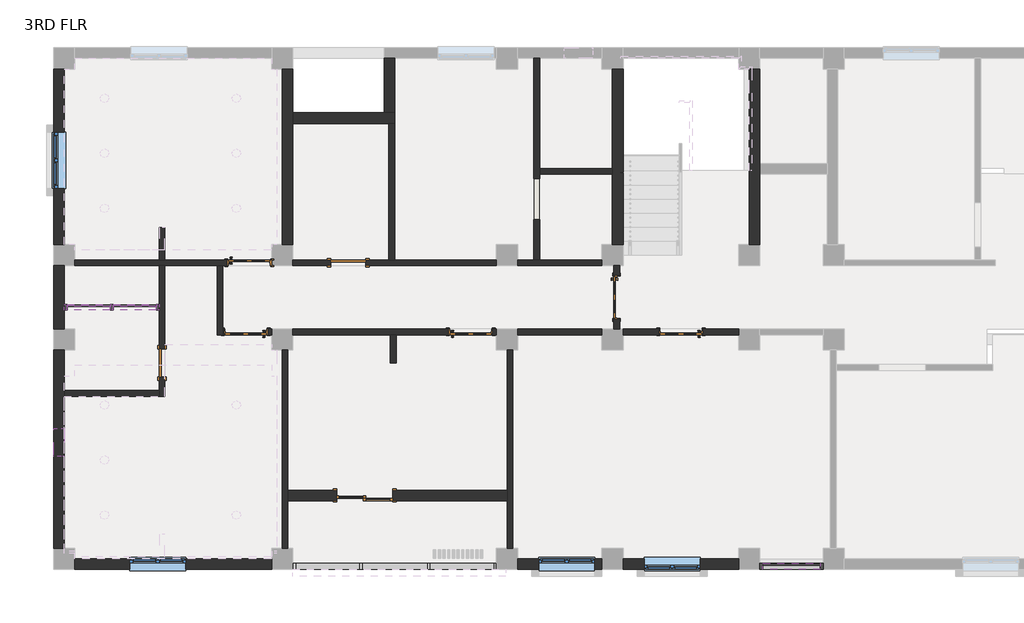
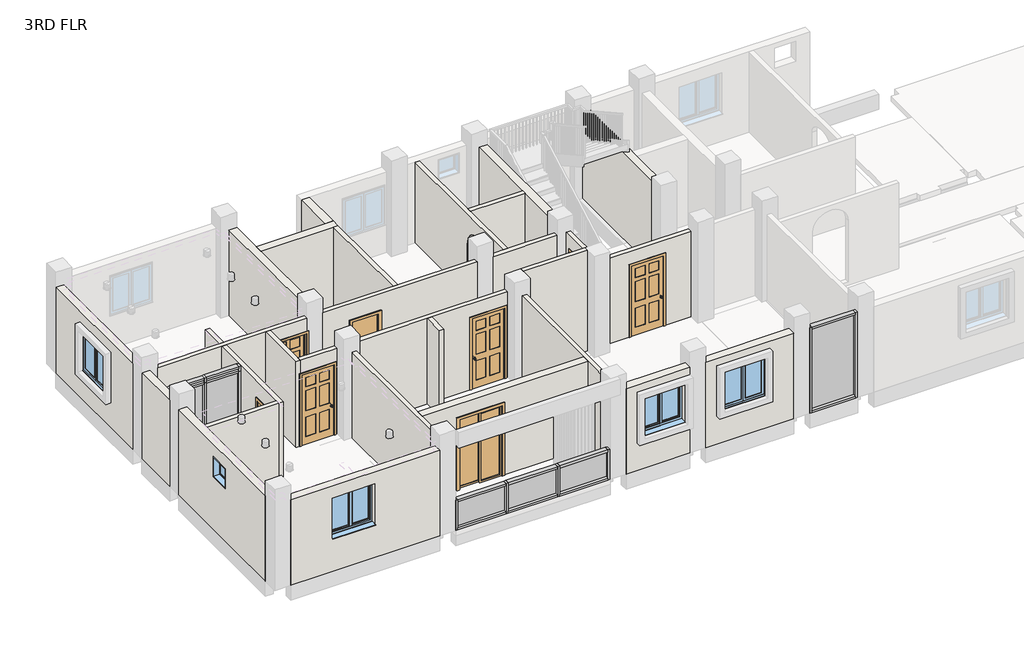
# One storey, part 1 of 5: 29 walls, 26 members, 8 doors, 8 plates, 5 windows.
"""IFC4 building model written with IfcOpenShell, lengths in millimetres."""

from ifc_helpers import new_model, si_unit, point, frame, origin, place, context, project, spatial, polyline, ellipse_curve, trimmed, outline, extrude, faceted_brep, transform, mapped, element, save
from ifc_brep_helpers import plane_surface, extruded_surface, advanced_brep
from components import door_double_sliding_4436dcad, door_c610b25b, door_03e3dfb5, single_flush_2_x_7_bath_room_door_025d1c86, door_e00f436c, member_f0fea5a5, member_f6f0dfdd, member_ee409385, member_876f8f00, member_2b4cd6f1, member_0dc43c0c, member_51239652, member_c58de4df, member_410c6227, member_73c23c35, member_71eb4692, member_9f3fc137, system_panel_glazed_e8343dfa, system_panel_glazed_58efc156, system_panel_glazed_69a0d9e9, system_panel_glazed_27716cba, system_panel_glazed_7ffa2d15, window_80340324, w2_0001_4_x_4_window_9dec5fc7

model = new_model("IFC4")

# Units and contexts
model_context = context("Model", 3, world=origin())
ifc_project = project(units=[si_unit("LENGTHUNIT", "METRE", prefix="MILLI")], contexts=[model_context])

# Site, building, storey
site = spatial("IfcSite", under=ifc_project)
building = spatial("IfcBuilding", under=site)
storey = spatial("IfcBuildingStorey", under=building, Name="3RD FLR", Elevation=9448.8)

# Doors
placement = place(None, origin())
door_double_sliding_shape = door_double_sliding_4436dcad(model_context)
element("IfcDoor", 1, ObjectType="Door-Double-Sliding", at=placement, inside=storey, context=model_context, shape_type="MappedRepresentation", body=[
    mapped(door_double_sliding_shape, transform((-8630.2456086, -9389.2679047, 9448.8), x_axis=(-1.0, 0.0, 0.0), y_axis=(0.0, -1.0, 0.0), z_axis=(0.0, 0.0, 1.0))),
])
door_shape = door_c610b25b(model_context)
element("IfcDoor", 2, ObjectType="Door-Interior-Single-6_Panel-Wood : 36\" x 84\"", at=placement, inside=storey, context=model_context, shape_type="MappedRepresentation", body=[
    mapped(door_shape, transform((-6331.5456086, -5967.8544704, 9448.8), x_axis=(1.0, 0.0, 0.0), y_axis=(0.0, 1.0, 0.0), z_axis=(0.0, 0.0, 1.0))),
])
element("IfcDoor", 3, ObjectType="Door-Interior-Single-6_Panel-Wood : 36\" x 84\"", at=placement, inside=storey, context=model_context, shape_type="MappedRepresentation", body=[
    mapped(door_shape, transform((-3172.4206086, -5215.3794704, 9448.8), x_axis=(0.0, -1.0, 0.0), y_axis=(1.0, 0.0, 0.0), z_axis=(0.0, 0.0, 1.0))),
])
door_2_shape = door_03e3dfb5(model_context)
element("IfcDoor", 4, ObjectType="Door-Interior-Single-6_Panel-Wood : 36\" x 84\"", at=placement, inside=storey, context=model_context, shape_type="MappedRepresentation", body=[
    mapped(door_2_shape, transform((-11207.742897, -5967.8544704, 9448.8), x_axis=(-1.0, 0.0, 0.0), y_axis=(0.0, -1.0, 0.0), z_axis=(0.0, 0.0, 1.0))),
])
element("IfcDoor", 5, ObjectType="Door-Interior-Single-6_Panel-Wood : 36\" x 84\"", at=placement, inside=storey, context=model_context, shape_type="MappedRepresentation", body=[
    mapped(door_2_shape, transform((-11132.1456086, -4462.9044704, 9448.8), x_axis=(1.0, 0.0, 0.0), y_axis=(0.0, 1.0, 0.0), z_axis=(0.0, 0.0, 1.0))),
])
element("IfcDoor", 6, ObjectType="Door-Interior-Single-6_Panel-Wood : 36\" x 84\"", at=placement, inside=storey, context=model_context, shape_type="MappedRepresentation", body=[
    mapped(door_2_shape, transform((-1773.9769742, -5967.8544704, 9448.8), x_axis=(-1.0, 0.0, 0.0), y_axis=(0.0, -1.0, 0.0), z_axis=(0.0, 0.0, 1.0))),
])
single_flush_2_x_7_bath_room_door_shape = single_flush_2_x_7_bath_room_door_025d1c86(model_context)
element("IfcDoor", 7, ObjectType="Single-Flush : 2' X 7' BATH ROOM DOOR", at=placement, inside=storey, context=model_context, shape_type="MappedRepresentation", body=[
    mapped(single_flush_2_x_7_bath_room_door_shape, transform((-13023.2401855, -6639.2659448, 9448.8), x_axis=(0.0, 1.0, 0.0), y_axis=(-1.0, 0.0, 0.0), z_axis=(0.0, 0.0, 1.0))),
])
door_3_shape = door_e00f436c(model_context)
element("IfcDoor", 8, ObjectType="Single-Flush : bathroom 2'6\" door", at=placement, inside=storey, context=model_context, shape_type="MappedRepresentation", body=[
    mapped(door_3_shape, transform((-8985.8456086, -4466.0794704, 9448.8), x_axis=(-1.0, 0.0, 0.0), y_axis=(0.0, -1.0, 0.0), z_axis=(0.0, 0.0, 1.0))),
])

# Members
member_shape = member_f0fea5a5(model_context)
element("IfcMember", 9, ObjectType="Rectangular Mullion : 2.5\" x 5\" rectangular", at=placement, inside=storey, context=model_context, shape_type="MappedRepresentation", body=[
    mapped(member_shape, transform((-14116.042897, -5431.2794704, 9448.8), x_axis=(1.0, 0.0, 0.0), y_axis=(0.0, -1.0, 0.0), z_axis=(0.0, 0.0, -1.0))),
])
member_2_shape = member_f6f0dfdd(model_context)
element("IfcMember", 10, ObjectType="Rectangular Mullion : 2.5\" x 5\" rectangular", at=placement, inside=storey, context=model_context, shape_type="MappedRepresentation", body=[
    mapped(member_2_shape, transform((-14116.042897, -5431.2794704, 11887.2), x_axis=(1.0, 0.0, 0.0), y_axis=(0.0, -1.0, 0.0), z_axis=(0.0, 0.0, -1.0))),
])
member_3_shape = member_ee409385(model_context)
element("IfcMember", 11, ObjectType="Rectangular Mullion : 2.5\" x 5\" rectangular", at=placement, inside=storey, context=model_context, shape_type="MappedRepresentation", body=[
    mapped(member_3_shape, transform((-13086.7401855, -5431.2794704, 9448.8), x_axis=(1.0, 0.0, 0.0), y_axis=(0.0, -1.0, 0.0), z_axis=(0.0, 0.0, -1.0))),
])
member_4_shape = member_876f8f00(model_context)
element("IfcMember", 12, ObjectType="Rectangular Mullion : 2.5\" x 5\" rectangular", at=placement, inside=storey, context=model_context, shape_type="MappedRepresentation", body=[
    mapped(member_4_shape, transform((-15145.3456086, -5431.2794704, 12039.6), x_axis=(-1.0, 0.0, 0.0), y_axis=(0.0, -1.0, 0.0), z_axis=(0.0, 0.0, 1.0))),
])
element("IfcMember", 13, ObjectType="Rectangular Mullion : 2.5\" x 5\" rectangular", at=placement, inside=storey, context=model_context, shape_type="MappedRepresentation", body=[
    mapped(member_4_shape, transform((-13086.7401855, -5431.2794704, 11887.2), x_axis=(1.0, 0.0, 0.0), y_axis=(0.0, -1.0, 0.0), z_axis=(0.0, 0.0, -1.0))),
])
element("IfcMember", 14, ObjectType="Rectangular Mullion : 2.5\" x 5\" rectangular", at=placement, inside=storey, context=model_context, shape_type="MappedRepresentation", body=[
    mapped(member_3_shape, transform((-15145.3456086, -5431.2794704, 11887.2), x_axis=(-1.0, 0.0, 0.0), y_axis=(0.0, -1.0, 0.0), z_axis=(0.0, 0.0, 1.0))),
])
member_5_shape = member_2b4cd6f1(model_context)
element("IfcMember", 15, ObjectType="Rectangular Mullion : 2.5\" x 5\" rectangular", at=placement, inside=storey, context=model_context, shape_type="MappedRepresentation", body=[
    mapped(member_5_shape, transform((-5836.2456086, -11052.9679047, 10363.2), x_axis=(0.0, 0.0, 1.0), y_axis=(0.0, -1.0, 0.0), z_axis=(1.0, 0.0, 0.0))),
])
element("IfcMember", 16, ObjectType="Rectangular Mullion : 2.5\" x 5\" rectangular", at=placement, inside=storey, context=model_context, shape_type="MappedRepresentation", body=[
    mapped(member_5_shape, transform((-8750.8956085, -11052.9679047, 10363.2), x_axis=(0.0, 0.0, 1.0), y_axis=(0.0, -1.0, 0.0), z_axis=(1.0, 0.0, 0.0))),
])
element("IfcMember", 17, ObjectType="Rectangular Mullion : 2.5\" x 5\" rectangular", at=placement, inside=storey, context=model_context, shape_type="MappedRepresentation", body=[
    mapped(member_5_shape, transform((-10128.8456086, -11052.9679047, 9448.8), x_axis=(0.0, 0.0, -1.0), y_axis=(0.0, -1.0, 0.0), z_axis=(-1.0, 0.0, 0.0))),
])
element("IfcMember", 18, ObjectType="Rectangular Mullion : 2.5\" x 5\" rectangular", at=placement, inside=storey, context=model_context, shape_type="MappedRepresentation", body=[
    mapped(member_5_shape, transform((-7214.1956087, -11052.9679047, 9448.8), x_axis=(0.0, 0.0, -1.0), y_axis=(0.0, -1.0, 0.0), z_axis=(-1.0, 0.0, 0.0))),
])
member_6_shape = member_0dc43c0c(model_context)
element("IfcMember", 19, ObjectType="Rectangular Mullion : 2.5\" x 5\" rectangular", at=placement, inside=storey, context=model_context, shape_type="MappedRepresentation", body=[
    mapped(member_6_shape, transform((-7277.6956087, -11052.9679047, 10363.2), x_axis=(0.0, 0.0, 1.0), y_axis=(0.0, -1.0, 0.0), z_axis=(1.0, 0.0, 0.0))),
])
element("IfcMember", 20, ObjectType="Rectangular Mullion : 2.5\" x 5\" rectangular", at=placement, inside=storey, context=model_context, shape_type="MappedRepresentation", body=[
    mapped(member_6_shape, transform((-8687.3956085, -11052.9679047, 9448.8), x_axis=(0.0, 0.0, -1.0), y_axis=(0.0, -1.0, 0.0), z_axis=(-1.0, 0.0, 0.0))),
])
member_7_shape = member_51239652(model_context)
element("IfcMember", 21, ObjectType="Rectangular Mullion : 2.5\" x 5\" rectangular", at=placement, inside=storey, context=model_context, shape_type="MappedRepresentation", body=[
    mapped(member_7_shape, transform((-13150.2401855, -5431.2794704, 12039.6), x_axis=(0.0, 0.0, 1.0), y_axis=(0.0, -1.0, 0.0), z_axis=(1.0, 0.0, 0.0))),
])
element("IfcMember", 22, ObjectType="Rectangular Mullion : 2.5\" x 5\" rectangular", at=placement, inside=storey, context=model_context, shape_type="MappedRepresentation", body=[
    mapped(member_7_shape, transform((-14147.792897, -5431.2794704, 12039.6), x_axis=(0.0, 0.0, 1.0), y_axis=(0.0, -1.0, 0.0), z_axis=(1.0, 0.0, 0.0))),
])
element("IfcMember", 23, ObjectType="Rectangular Mullion : 2.5\" x 5\" rectangular", at=placement, inside=storey, context=model_context, shape_type="MappedRepresentation", body=[
    mapped(member_7_shape, transform((-15081.8456086, -5431.2794704, 9448.8), x_axis=(0.0, 0.0, -1.0), y_axis=(0.0, -1.0, 0.0), z_axis=(-1.0, 0.0, 0.0))),
])
element("IfcMember", 24, ObjectType="Rectangular Mullion : 2.5\" x 5\" rectangular", at=placement, inside=storey, context=model_context, shape_type="MappedRepresentation", body=[
    mapped(member_7_shape, transform((-14084.292897, -5431.2794704, 9448.8), x_axis=(0.0, 0.0, -1.0), y_axis=(0.0, -1.0, 0.0), z_axis=(-1.0, 0.0, 0.0))),
])
member_8_shape = member_c58de4df(model_context)
element("IfcMember", 25, ObjectType="Rectangular Mullion : 2.5\" x 5\" rectangular", at=placement, inside=storey, context=model_context, shape_type="MappedRepresentation", body=[
    mapped(member_8_shape, transform((-14147.792897, -5431.2794704, 11887.2), x_axis=(0.0, 0.0, 1.0), y_axis=(0.0, -1.0, 0.0), z_axis=(1.0, 0.0, 0.0))),
])
element("IfcMember", 26, ObjectType="Rectangular Mullion : 2.5\" x 5\" rectangular", at=placement, inside=storey, context=model_context, shape_type="MappedRepresentation", body=[
    mapped(member_8_shape, transform((-13150.2401855, -5431.2794704, 11887.2), x_axis=(0.0, 0.0, 1.0), y_axis=(0.0, -1.0, 0.0), z_axis=(1.0, 0.0, 0.0))),
])
member_9_shape = member_410c6227(model_context)
element("IfcMember", 27, ObjectType="Rectangular Mullion : 2.5\" x 5\" rectangular", at=placement, inside=storey, context=model_context, shape_type="MappedRepresentation", body=[
    mapped(member_9_shape, transform((-8719.1456085, -11052.9679047, 9448.8), x_axis=(1.0, 0.0, 0.0), y_axis=(0.0, -1.0, 0.0), z_axis=(0.0, 0.0, -1.0))),
])
element("IfcMember", 28, ObjectType="Rectangular Mullion : 2.5\" x 5\" rectangular", at=placement, inside=storey, context=model_context, shape_type="MappedRepresentation", body=[
    mapped(member_9_shape, transform((-7245.9456087, -11052.9679047, 9448.8), x_axis=(1.0, 0.0, 0.0), y_axis=(0.0, -1.0, 0.0), z_axis=(0.0, 0.0, -1.0))),
])
member_10_shape = member_73c23c35(model_context)
element("IfcMember", 29, ObjectType="Rectangular Mullion : 2.5\" x 5\" rectangular", at=placement, inside=storey, context=model_context, shape_type="MappedRepresentation", body=[
    mapped(member_10_shape, transform((-5772.7456086, -11052.9679047, 9448.8), x_axis=(1.0, 0.0, 0.0), y_axis=(0.0, -1.0, 0.0), z_axis=(0.0, 0.0, -1.0))),
])
element("IfcMember", 30, ObjectType="Rectangular Mullion : 2.5\" x 5\" rectangular", at=placement, inside=storey, context=model_context, shape_type="MappedRepresentation", body=[
    mapped(member_10_shape, transform((-10192.3456086, -11052.9679047, 10363.2), x_axis=(-1.0, 0.0, 0.0), y_axis=(0.0, -1.0, 0.0), z_axis=(0.0, 0.0, 1.0))),
])
member_11_shape = member_71eb4692(model_context)
element("IfcMember", 31, ObjectType="Rectangular Mullion : 2.5\" x 5\" rectangular", at=placement, inside=storey, context=model_context, shape_type="MappedRepresentation", body=[
    mapped(member_11_shape, transform((1246.8916602, -11052.9679047, 12039.6), x_axis=(0.0, 0.0, 1.0), y_axis=(0.0, -1.0, 0.0), z_axis=(1.0, 0.0, 0.0))),
])
element("IfcMember", 32, ObjectType="Rectangular Mullion : 2.5\" x 5\" rectangular", at=placement, inside=storey, context=model_context, shape_type="MappedRepresentation", body=[
    mapped(member_11_shape, transform((2.2916602, -11052.9679047, 9448.8), x_axis=(0.0, 0.0, -1.0), y_axis=(0.0, -1.0, 0.0), z_axis=(-1.0, 0.0, 0.0))),
])
member_12_shape = member_9f3fc137(model_context)
element("IfcMember", 33, ObjectType="Rectangular Mullion : 2.5\" x 5\" rectangular", at=placement, inside=storey, context=model_context, shape_type="MappedRepresentation", body=[
    mapped(member_12_shape, transform((1310.3916602, -11052.9679047, 9448.8), x_axis=(1.0, 0.0, 0.0), y_axis=(0.0, -1.0, 0.0), z_axis=(0.0, 0.0, -1.0))),
])
element("IfcMember", 34, ObjectType="Rectangular Mullion : 2.5\" x 5\" rectangular", at=placement, inside=storey, context=model_context, shape_type="MappedRepresentation", body=[
    mapped(member_12_shape, transform((-61.2083398, -11052.9679047, 12039.6), x_axis=(-1.0, 0.0, 0.0), y_axis=(0.0, -1.0, 0.0), z_axis=(0.0, 0.0, 1.0))),
])

# Plates
system_panel_glazed_shape = system_panel_glazed_e8343dfa(model_context)
element("IfcPlate", 35, ObjectType="System Panel : Glazed", at=placement, inside=storey, context=model_context, shape_type="MappedRepresentation", body=[
    mapped(system_panel_glazed_shape, transform((-14614.8192528, -5431.2794704, 9512.3), x_axis=(1.0, 0.0, 0.0), y_axis=(0.0, 1.0, 0.0), z_axis=(0.0, 0.0, 1.0))),
])
element("IfcPlate", 36, ObjectType="System Panel : Glazed", at=placement, inside=storey, context=model_context, shape_type="MappedRepresentation", body=[
    mapped(system_panel_glazed_shape, transform((-13617.2665413, -5431.2794704, 9512.3), x_axis=(1.0, 0.0, 0.0), y_axis=(0.0, 1.0, 0.0), z_axis=(0.0, 0.0, 1.0))),
])
system_panel_glazed_2_shape = system_panel_glazed_58efc156(model_context)
element("IfcPlate", 37, ObjectType="System Panel : Glazed", at=placement, inside=storey, context=model_context, shape_type="MappedRepresentation", body=[
    mapped(system_panel_glazed_2_shape, transform((-14614.8192528, -5431.2794704, 11918.95), x_axis=(1.0, 0.0, 0.0), y_axis=(0.0, 1.0, 0.0), z_axis=(0.0, 0.0, 1.0))),
])
element("IfcPlate", 38, ObjectType="System Panel : Glazed", at=placement, inside=storey, context=model_context, shape_type="MappedRepresentation", body=[
    mapped(system_panel_glazed_2_shape, transform((-13617.2665413, -5431.2794704, 11918.95), x_axis=(1.0, 0.0, 0.0), y_axis=(0.0, 1.0, 0.0), z_axis=(0.0, 0.0, 1.0))),
])
system_panel_glazed_3_shape = system_panel_glazed_69a0d9e9(model_context)
element("IfcPlate", 39, ObjectType="System Panel : Glazed", at=placement, inside=storey, context=model_context, shape_type="MappedRepresentation", body=[
    mapped(system_panel_glazed_3_shape, transform((-9439.8706086, -11052.9679047, 9512.3), x_axis=(1.0, 0.0, 0.0), y_axis=(0.0, 1.0, 0.0), z_axis=(0.0, 0.0, 1.0))),
])
element("IfcPlate", 40, ObjectType="System Panel : Glazed", at=placement, inside=storey, context=model_context, shape_type="MappedRepresentation", body=[
    mapped(system_panel_glazed_3_shape, transform((-6525.2206087, -11052.9679047, 9512.3), x_axis=(1.0, 0.0, 0.0), y_axis=(0.0, 1.0, 0.0), z_axis=(0.0, 0.0, 1.0))),
])
system_panel_glazed_4_shape = system_panel_glazed_27716cba(model_context)
element("IfcPlate", 41, ObjectType="System Panel : Glazed", at=placement, inside=storey, context=model_context, shape_type="MappedRepresentation", body=[
    mapped(system_panel_glazed_4_shape, transform((-7982.5456086, -11052.9679047, 9512.3), x_axis=(1.0, 0.0, 0.0), y_axis=(0.0, 1.0, 0.0), z_axis=(0.0, 0.0, 1.0))),
])
system_panel_glazed_5_shape = system_panel_glazed_7ffa2d15(model_context)
element("IfcPlate", 42, ObjectType="System Panel : Glazed", at=placement, inside=storey, context=model_context, shape_type="MappedRepresentation", body=[
    mapped(system_panel_glazed_5_shape, transform((624.5916602, -11052.9679047, 9512.3), x_axis=(1.0, 0.0, 0.0), y_axis=(0.0, 1.0, 0.0), z_axis=(0.0, 0.0, 1.0))),
])

# Walls
element("IfcWall", 43, ObjectType="EXTERIOR WALL 9\"", at=placement, inside=storey, context=model_context, shape_type="SweptSolid", body=[
    extrude(outline(polyline([(9448.8, -14916.7456086), (9448.8, -10649.5456086), (12039.6, -10649.5456086), (12039.6, -14916.7456086), (9448.8, -14916.7456086)]), holes=[polyline([(10448.8, -12503.7456086), (10448.8, -13722.9456086), (11668.0, -13722.9456086), (11668.0, -12503.7456086), (10448.8, -12503.7456086)])]), frame((0.0, -11116.4679047, 0.0), z_axis=(0.0, 1.0, 0.0), x_axis=(0.0, 0.0, 1.0)), (0.0, 0.0, 1.0), 228.6),
])
element("IfcWall", 44, ObjectType="EXTERIOR WALL 9\"", at=placement, inside=storey, context=model_context, shape_type="SweptSolid", body=[
    extrude(outline(polyline([(9448.8, -5315.5456086), (9448.8, -3486.7456086), (12039.6, -3486.7456086), (12039.6, -5315.5456086), (9448.8, -5315.5456086)]), holes=[polyline([(10448.8, -3639.1456086), (10448.8, -4858.3456086), (11668.0, -4858.3456086), (11668.0, -3639.1456086), (10448.8, -3639.1456086)])]), frame((0.0, -11116.4679047, 0.0), z_axis=(0.0, 1.0, 0.0), x_axis=(0.0, 0.0, 1.0)), (0.0, 0.0, 1.0), 228.6),
])
element("IfcWall", 45, ObjectType="EXTERIOR WALL 9\"", at=placement, inside=storey, context=model_context, shape_type="SweptSolid", body=[
    extrude(outline(polyline([(9448.8, -3029.5456086), (9448.8, -518.4083398), (12039.6, -518.4083398), (12039.6, -3029.5456086), (9448.8, -3029.5456086)]), holes=[polyline([(10448.8, -2572.3456086), (11668.0, -2572.3456086), (11668.0, -1353.1456086), (10448.8, -1353.1456086), (10448.8, -2572.3456086)])]), frame((0.0, -11116.4679047, 0.0), z_axis=(0.0, 1.0, 0.0), x_axis=(0.0, 0.0, 1.0)), (0.0, 0.0, 1.0), 228.6),
])
element("IfcWall", 46, ObjectType="EXTERIOR WALL 9\"", at=placement, inside=storey, context=model_context, shape_type="Brep", body=[
    faceted_brep([(-15145.3456086, -10659.2679047, 9448.8), (-15145.3456086, -7363.1659448, 9448.8), (-15145.3456086, -7236.1659448, 9448.8), (-15145.3456086, -6358.3794704, 9448.8), (-15145.3456086, -6358.3794704, 12039.6), (-15145.3456086, -7236.1659448, 12039.6), (-15145.3456086, -7363.1659448, 12039.6), (-15145.3456086, -10659.2679047, 12039.6), (-15145.3456086, -8671.2659448, 11655.8263913), (-15145.3456086, -8061.6659448, 11655.8263913), (-15145.3456086, -8061.6659448, 11046.2263913), (-15145.3456086, -8671.2659448, 11046.2263913), (-15373.9456086, -10659.2679047, 9448.8), (-15373.9456086, -10659.2679047, 12039.6), (-15373.9456086, -6358.3794704, 12039.6), (-15373.9456086, -6358.3794704, 9448.8), (-15373.9456086, -8671.2659448, 11655.8263913), (-15373.9456086, -8671.2659448, 11046.2263913), (-15373.9456086, -8061.6659448, 11046.2263913), (-15373.9456086, -8061.6659448, 11655.8263913)], [[[0, 1, 2, 3, 4, 5, 6, 7], [8, 9, 10, 11]], [[12, 13, 14, 15], [16, 17, 18, 19]], [[3, 2, 1, 0, 12, 15]], [[4, 3, 15, 14]], [[7, 6, 5, 4, 14, 13]], [[0, 7, 13, 12]], [[17, 16, 8, 11]], [[18, 17, 11, 10]], [[19, 18, 10, 9]], [[16, 19, 9, 8]]]),
])
element("IfcWall", 47, ObjectType="EXTERIOR WALL 9\"", at=placement, inside=storey, context=model_context, shape_type="SweptSolid", body=[
    extrude(outline(polyline([(-15145.3456086, -4529.5794704), (-15145.3456086, -5901.1794704), (-15373.9456086, -5901.1794704), (-15373.9456086, -4529.5794704), (-15145.3456086, -4529.5794704)])), frame((0.0, 0.0, 9448.8), z_axis=(0.0, 0.0, 1.0), x_axis=(1.0, 0.0, 0.0)), (0.0, 0.0, 1.0), 2590.8),
])
element("IfcWall", 48, ObjectType="EXTERIOR WALL 9\"", at=placement, inside=storey, context=model_context, shape_type="SweptSolid", body=[
    extrude(outline(polyline([(-262.3794704, 9448.8), (-4072.3794704, 9448.8), (-4072.3794704, 12039.6), (-262.3794704, 12039.6), (-262.3794704, 9448.8)]), holes=[polyline([(-1633.9794704, 10363.2), (-1633.9794704, 11582.4), (-2853.1794704, 11582.4), (-2853.1794704, 10363.2), (-1633.9794704, 10363.2)])]), frame((-15373.9456086, 0.0, 0.0), z_axis=(1.0, 0.0, 0.0), x_axis=(0.0, 1.0, 0.0)), (0.0, 0.0, 1.0), 228.6),
])
element("IfcWall", 49, ObjectType="EXTERIOR WALL 9\"", at=placement, inside=storey, context=model_context, shape_type="Brep", body=[
    faceted_brep([(-10420.9456086, -262.3794704, 9448.8), (-10420.9456086, -4072.3794704, 9448.8), (-10420.9456086, -4072.3794704, 12039.6), (-10420.9456086, -262.3794704, 12039.6), (-10192.3456086, -262.3794704, 9448.8), (-10192.3456086, -262.3794704, 12039.6), (-10192.3456086, -1214.8794704, 12039.6), (-10192.3456086, -1443.4794704, 12039.6), (-10192.3456086, -4072.3794704, 12039.6), (-10192.3456086, -4072.3794704, 9448.8), (-10192.3456086, -1443.4794704, 9448.8), (-10192.3456086, -1214.8794704, 9448.8)], [[[0, 1, 2, 3]], [[4, 5, 6, 7, 8, 9, 10, 11]], [[1, 0, 4, 11, 10, 9]], [[2, 1, 9, 8]], [[3, 2, 8, 7, 6, 5]], [[0, 3, 5, 4]]]),
])
element("IfcWall", 50, ObjectType="EXTERIOR WALL 9\"", at=placement, inside=storey, context=model_context, shape_type="SweptSolid", body=[
    extrude(outline(polyline([(9448.8, -10293.9456086), (9448.8, -9239.8456086), (11582.4, -9239.8456086), (11582.4, -8020.6456086), (9448.8, -8020.6456086), (9448.8, -5544.1456086), (12039.6, -5544.1456086), (12039.6, -10293.9456086), (9448.8, -10293.9456086)])), frame((0.0, -9630.5679047, 0.0), z_axis=(0.0, 1.0, 0.0), x_axis=(0.0, 0.0, 1.0)), (0.0, 0.0, 1.0), 228.6),
])
element("IfcWall", 51, ObjectType="EXTERIOR WALL 9\"", at=placement, inside=storey, context=model_context, shape_type="Brep", body=[
    faceted_brep([(-10192.3456086, -1443.4794704, 9448.8), (-8109.5456086, -1443.4794704, 9448.8), (-7982.5456086, -1443.4794704, 9448.8), (-7982.5456086, -1443.4794704, 12039.6), (-8109.5456086, -1443.4794704, 12039.6), (-10192.3456086, -1443.4794704, 12039.6), (-10192.3456086, -1214.8794704, 9448.8), (-10192.3456086, -1214.8794704, 12039.6), (-8211.1456086, -1214.8794704, 12039.6), (-7982.5456086, -1214.8794704, 12039.6), (-7982.5456086, -1214.8794704, 9448.8), (-8211.1456086, -1214.8794704, 9448.8)], [[[0, 1, 2, 3, 4, 5]], [[6, 7, 8, 9, 10, 11]], [[2, 1, 0, 6, 11, 10]], [[5, 4, 3, 9, 8, 7]], [[0, 5, 7, 6]], [[3, 2, 10, 9]]]),
])
element("IfcWall", 52, ObjectType="EXTERIOR WALL 9\"", at=placement, inside=storey, context=model_context, shape_type="SweptSolid", body=[
    extrude(outline(polyline([(-7982.5456086, -33.7794704), (-7982.5456086, -1214.8794704), (-8211.1456086, -1214.8794704), (-8211.1456086, -33.7794704), (-7982.5456086, -33.7794704)])), frame((0.0, 0.0, 9448.8), z_axis=(0.0, 0.0, 1.0), x_axis=(1.0, 0.0, 0.0)), (0.0, 0.0, 1.0), 2590.8),
])
element("IfcWall", 53, ObjectType="EXTERIOR WALL 9\"", at=placement, inside=storey, context=model_context, shape_type="Brep", body=[
    faceted_brep([(-3258.1456086, -262.3794704, 9448.8), (-3258.1456086, -2421.3794704, 9448.8), (-3258.1456086, -2548.3794704, 9448.8), (-3258.1456086, -4072.3794704, 9448.8), (-3258.1456086, -4072.3794704, 12039.6), (-3258.1456086, -2548.3794704, 12039.6), (-3258.1456086, -2421.3794704, 12039.6), (-3258.1456086, -262.3794704, 12039.6), (-3029.5456086, -262.3794704, 9448.8), (-3029.5456086, -262.3794704, 12039.6), (-3029.5456086, -4072.3794704, 12039.6), (-3029.5456086, -4072.3794704, 9448.8)], [[[0, 1, 2, 3, 4, 5, 6, 7]], [[8, 9, 10, 11]], [[3, 2, 1, 0, 8, 11]], [[4, 3, 11, 10]], [[7, 6, 5, 4, 10, 9]], [[0, 7, 9, 8]]]),
])
element("IfcWall", 54, ObjectType="EXTERIOR WALL 9\"", at=placement, inside=storey, context=model_context, shape_type="Brep", body=[
    faceted_brep([(-289.8083398, -262.3794704, 9448.8), (-289.8083398, -4072.3794704, 9448.8), (-289.8083398, -4072.3794704, 12039.6), (-289.8083398, -262.3794704, 12039.6), (-61.2083398, -262.3794704, 9448.8), (-61.2083398, -262.3794704, 12039.6), (-61.2083398, -2319.7794704, 12039.6), (-61.2083398, -2548.3794704, 12039.6), (-61.2083398, -4072.3794704, 12039.6), (-61.2083398, -4072.3794704, 9448.8), (-61.2083398, -2548.3794704, 9448.8), (-61.2083398, -2319.7794704, 9448.8)], [[[0, 1, 2, 3]], [[4, 5, 6, 7, 8, 9, 10, 11]], [[1, 0, 4, 11, 10, 9]], [[2, 1, 9, 8]], [[3, 2, 8, 7, 6, 5]], [[0, 3, 5, 4]]]),
])
element("IfcWall", 55, ObjectType="INTERIOR WALL 5\"", at=placement, inside=storey, context=model_context, shape_type="Brep", body=[
    faceted_brep([(-10649.5456086, -4529.5794704, 12039.6), (-11702.4401855, -4529.5794704, 12039.6), (-11829.4401855, -4529.5794704, 12039.6), (-12959.7401855, -4529.5794704, 12039.6), (-13086.7401855, -4529.5794704, 12039.6), (-14916.7456086, -4529.5794704, 12039.6), (-14916.7456086, -4529.5794704, 9448.8), (-13086.7401855, -4529.5794704, 9448.8), (-12959.7401855, -4529.5794704, 9448.8), (-11829.4401855, -4529.5794704, 9448.8), (-11702.4401855, -4529.5794704, 9448.8), (-11614.7456086, -4529.5794704, 9448.8), (-11614.7456086, -4529.5794704, 11607.8), (-10649.5456086, -4529.5794704, 11607.8), (-14916.7456086, -4402.5794704, 12039.6), (-13086.7401855, -4402.5794704, 12039.6), (-12959.7401855, -4402.5794704, 12039.6), (-10649.5456086, -4402.5794704, 12039.6), (-10649.5456086, -4402.5794704, 11607.8), (-11614.7456086, -4402.5794704, 11607.8), (-11614.7456086, -4402.5794704, 9448.8), (-12959.7401855, -4402.5794704, 9448.8), (-13086.7401855, -4402.5794704, 9448.8), (-14916.7456086, -4402.5794704, 9448.8)], [[[0, 1, 2, 3, 4, 5, 6, 7, 8, 9, 10, 11, 12, 13]], [[14, 15, 16, 17, 18, 19, 20, 21, 22, 23]], [[6, 23, 22, 21, 20, 11, 10, 9, 8, 7]], [[17, 0, 13, 18]], [[5, 4, 3, 2, 1, 0, 17, 16, 15, 14]], [[6, 5, 14, 23]], [[12, 19, 18, 13]], [[19, 12, 11, 20]]]),
])
element("IfcWall", 56, ObjectType="INTERIOR WALL 5\"", at=placement, inside=storey, context=model_context, shape_type="Brep", body=[
    faceted_brep([(-13086.7401855, -3705.5659448, 12039.6), (-13086.7401855, -3705.5659448, 9448.8), (-13086.7401855, -4402.5794704, 9448.8), (-13086.7401855, -4402.5794704, 12039.6), (-12959.7401855, -3705.5659448, 9448.8), (-12959.7401855, -3705.5659448, 12039.6), (-12959.7401855, -4402.5794704, 12039.6), (-12959.7401855, -4402.5794704, 9448.8)], [[[0, 1, 2, 3]], [[4, 5, 6, 7]], [[1, 4, 7, 2]], [[5, 0, 3, 6]], [[1, 0, 5, 4]], [[3, 2, 7, 6]]]),
    faceted_brep([(-13086.7401855, -7363.1659448, 9448.8), (-13086.7401855, -7363.1659448, 12039.6), (-13086.7401855, -7236.1659448, 12039.6), (-13086.7401855, -4529.5794704, 12039.6), (-13086.7401855, -4529.5794704, 9448.8), (-13086.7401855, -6334.4659448, 9448.8), (-13086.7401855, -6334.4659448, 11480.8), (-13086.7401855, -6944.0659448, 11480.8), (-13086.7401855, -6944.0659448, 9448.8), (-13086.7401855, -7236.1659448, 9448.8), (-12959.7401855, -7363.1659448, 12039.6), (-12959.7401855, -7363.1659448, 9448.8), (-12959.7401855, -6944.0659448, 9448.8), (-12959.7401855, -6944.0659448, 11480.8), (-12959.7401855, -6334.4659448, 11480.8), (-12959.7401855, -6334.4659448, 9448.8), (-12959.7401855, -4529.5794704, 9448.8), (-12959.7401855, -4529.5794704, 12039.6)], [[[0, 1, 2, 3, 4, 5, 6, 7, 8, 9]], [[10, 11, 12, 13, 14, 15, 16, 17]], [[11, 0, 9, 8, 12]], [[15, 5, 4, 16]], [[1, 10, 17, 3, 2]], [[4, 3, 17, 16]], [[1, 0, 11, 10]], [[6, 5, 15, 14]], [[7, 6, 14, 13]], [[8, 7, 13, 12]]]),
])
element("IfcWall", 57, ObjectType="INTERIOR WALL 5\"", at=placement, inside=storey, context=model_context, shape_type="SweptSolid", body=[
    extrude(outline(polyline([(-15145.3456086, -7236.1659448), (-13086.7401855, -7236.1659448), (-13086.7401855, -7363.1659448), (-15145.3456086, -7363.1659448), (-15145.3456086, -7236.1659448)])), frame((0.0, 0.0, 9448.8), z_axis=(0.0, 0.0, 1.0), x_axis=(1.0, 0.0, 0.0)), (0.0, 0.0, 1.0), 2590.8),
])
element("IfcWall", 58, ObjectType="INTERIOR WALL 5\"", at=placement, inside=storey, context=model_context, shape_type="Brep", body=[
    faceted_brep([(-10293.9456086, -10659.2679047, 9448.8), (-10293.9456086, -9630.5679047, 9448.8), (-10293.9456086, -9401.9679047, 9448.8), (-10293.9456086, -6358.3794704, 9448.8), (-10293.9456086, -6358.3794704, 12039.6), (-10293.9456086, -9401.9679047, 12039.6), (-10293.9456086, -9630.5679047, 12039.6), (-10293.9456086, -10659.2679047, 12039.6), (-10420.9456086, -10659.2679047, 9448.8), (-10420.9456086, -10659.2679047, 12039.6), (-10420.9456086, -6358.3794704, 12039.6), (-10420.9456086, -6358.3794704, 9448.8)], [[[0, 1, 2, 3, 4, 5, 6, 7]], [[8, 9, 10, 11]], [[3, 2, 1, 0, 8, 11]], [[4, 3, 11, 10]], [[7, 6, 5, 4, 10, 9]], [[0, 7, 9, 8]]]),
])
element("IfcWall", 59, ObjectType="INTERIOR WALL 5\"", at=placement, inside=storey, context=model_context, shape_type="Brep", body=[
    faceted_brep([(-10192.3456086, -5901.1794704, 9448.8), (-10192.3456086, -5901.1794704, 12039.6), (-5772.7456086, -5901.1794704, 12039.6), (-5772.7456086, -5901.1794704, 9448.8), (-5848.9456086, -5901.1794704, 9448.8), (-5848.9456086, -5901.1794704, 11607.8), (-6814.1456086, -5901.1794704, 11607.8), (-6814.1456086, -5901.1794704, 9448.8), (-10192.3456086, -6028.1794704, 12039.6), (-10192.3456086, -6028.1794704, 9448.8), (-8071.4456086, -6028.1794704, 9448.8), (-7944.4456086, -6028.1794704, 9448.8), (-6814.1456086, -6028.1794704, 9448.8), (-6814.1456086, -6028.1794704, 11607.8), (-5848.9456086, -6028.1794704, 11607.8), (-5848.9456086, -6028.1794704, 9448.8), (-5772.7456086, -6028.1794704, 9448.8), (-5772.7456086, -6028.1794704, 12039.6), (-7944.4456086, -6028.1794704, 12039.6), (-8071.4456086, -6028.1794704, 12039.6)], [[[0, 1, 2, 3, 4, 5, 6, 7]], [[8, 9, 10, 11, 12, 13, 14, 15, 16, 17, 18, 19]], [[9, 0, 7, 12, 11, 10]], [[3, 16, 15, 4]], [[1, 0, 9, 8]], [[2, 1, 8, 19, 18, 17]], [[3, 2, 17, 16]], [[14, 5, 4, 15]], [[5, 14, 13, 6]], [[6, 13, 12, 7]]]),
])
element("IfcWall", 60, ObjectType="INTERIOR WALL 5\"", at=placement, inside=storey, context=model_context, shape_type="SweptSolid", body=[
    extrude(outline(polyline([(-8071.4456086, -6637.7794704), (-8071.4456086, -6028.1794704), (-7944.4456086, -6028.1794704), (-7944.4456086, -6637.7794704), (-8071.4456086, -6637.7794704)])), frame((0.0, 0.0, 9448.8), z_axis=(0.0, 0.0, 1.0), x_axis=(1.0, 0.0, 0.0)), (0.0, 0.0, 1.0), 2590.8),
])
element("IfcWall", 61, ObjectType="INTERIOR WALL 5\"", at=placement, inside=storey, context=model_context, shape_type="Brep", body=[
    faceted_brep([(-5417.1456086, -10659.2679047, 9448.8), (-5417.1456086, -6358.3794704, 9448.8), (-5417.1456086, -6358.3794704, 12039.6), (-5417.1456086, -10659.2679047, 12039.6), (-5544.1456086, -10659.2679047, 9448.8), (-5544.1456086, -10659.2679047, 12039.6), (-5544.1456086, -9630.5679047, 12039.6), (-5544.1456086, -9401.9679047, 12039.6), (-5544.1456086, -6358.3794704, 12039.6), (-5544.1456086, -6358.3794704, 9448.8), (-5544.1456086, -9401.9679047, 9448.8), (-5544.1456086, -9630.5679047, 9448.8)], [[[0, 1, 2, 3]], [[4, 5, 6, 7, 8, 9, 10, 11]], [[1, 0, 4, 11, 10, 9]], [[2, 1, 9, 8]], [[3, 2, 8, 7, 6, 5]], [[0, 3, 5, 4]]]),
])
element("IfcWall", 62, ObjectType="INTERIOR WALL 5\"", at=placement, inside=storey, context=model_context, shape_type="Brep", body=[
    faceted_brep([(-10192.3456086, -4529.5794704, 9448.8), (-9366.8456086, -4529.5794704, 9448.8), (-9366.8456086, -4529.5794704, 11480.8), (-8604.8456086, -4529.5794704, 11480.8), (-8604.8456086, -4529.5794704, 9448.8), (-5772.7456086, -4529.5794704, 9448.8), (-5772.7456086, -4529.5794704, 12039.6), (-10192.3456086, -4529.5794704, 12039.6), (-9366.8456086, -4402.5794704, 11480.8), (-9366.8456086, -4402.5794704, 9448.8), (-10192.3456086, -4402.5794704, 9448.8), (-10192.3456086, -4402.5794704, 12039.6), (-8109.5456086, -4402.5794704, 12039.6), (-7982.5456086, -4402.5794704, 12039.6), (-5772.7456086, -4402.5794704, 12039.6), (-5772.7456086, -4402.5794704, 9448.8), (-7982.5456086, -4402.5794704, 9448.8), (-8109.5456086, -4402.5794704, 9448.8), (-8604.8456086, -4402.5794704, 9448.8), (-8604.8456086, -4402.5794704, 11480.8)], [[[0, 1, 2, 3, 4, 5, 6, 7]], [[8, 9, 10, 11, 12, 13, 14, 15, 16, 17, 18, 19]], [[10, 9, 1, 0]], [[18, 17, 16, 15, 5, 4]], [[6, 5, 15, 14]], [[7, 6, 14, 13, 12, 11]], [[0, 7, 11, 10]], [[2, 1, 9, 8]], [[3, 2, 8, 19]], [[4, 3, 19, 18]]]),
])
element("IfcWall", 63, ObjectType="INTERIOR WALL 5\"", at=placement, inside=storey, context=model_context, shape_type="Brep", body=[
    faceted_brep([(-5315.5456086, -4529.5794704, 9448.8), (-3486.7456086, -4529.5794704, 9448.8), (-3486.7456086, -4529.5794704, 12039.6), (-5315.5456086, -4529.5794704, 12039.6), (-5315.5456086, -4402.5794704, 9448.8), (-5315.5456086, -4402.5794704, 12039.6), (-4959.9456086, -4402.5794704, 12039.6), (-4832.9456086, -4402.5794704, 12039.6), (-3486.7456086, -4402.5794704, 12039.6), (-3486.7456086, -4402.5794704, 9448.8), (-4832.9456086, -4402.5794704, 9448.8), (-4959.9456086, -4402.5794704, 9448.8)], [[[0, 1, 2, 3]], [[4, 5, 6, 7, 8, 9, 10, 11]], [[1, 0, 4, 11, 10, 9]], [[2, 1, 9, 8]], [[3, 2, 8, 7, 6, 5]], [[0, 3, 5, 4]]]),
])
element("IfcWall", 64, ObjectType="INTERIOR WALL 5\"", at=placement, inside=storey, context=model_context, shape_type="SweptSolid", body=[
    extrude(outline(polyline([(-8109.5456086, -4402.5794704), (-8109.5456086, -1443.4794704), (-7982.5456086, -1443.4794704), (-7982.5456086, -4402.5794704), (-8109.5456086, -4402.5794704)])), frame((0.0, 0.0, 9448.8), z_axis=(0.0, 0.0, 1.0), x_axis=(1.0, 0.0, 0.0)), (0.0, 0.0, 1.0), 2590.8),
])
element("IfcWall", 65, ObjectType="INTERIOR WALL 5\"", at=placement, inside=storey, context=model_context, shape_type="AdvancedBrep", body=[
    advanced_brep(
    [(-4959.9456086, -33.7794704, 9448.8), (-4959.9456086, -4402.5794704, 9448.8), (-4959.9456086, -4402.5794704, 12039.6), (-4959.9456086, -33.7794704, 12039.6), (-4959.9456086, -3525.9205586, 11137.0197979), (-4959.9456086, -3525.9205586, 9511.4197979), (-4959.9456086, -2636.9205586, 9511.4197979), (-4959.9456086, -2636.9205586, 11137.0197979), (-4832.9456086, -33.7794704, 9448.8), (-4832.9456086, -33.7794704, 12039.6), (-4832.9456086, -2421.3794704, 12039.6), (-4832.9456086, -2548.3794704, 12039.6), (-4832.9456086, -4402.5794704, 12039.6), (-4832.9456086, -4402.5794704, 9448.8), (-4832.9456086, -2548.3794704, 9448.8), (-4832.9456086, -2421.3794704, 9448.8), (-4832.9456086, -3525.9205586, 11137.0197979), (-4832.9456086, -2636.9205586, 11137.0197979), (-4832.9456086, -2636.9205586, 9511.4197979), (-4832.9456086, -3525.9205586, 9511.4197979)],
    [
        (0, 1),
        (1, 2),
        (2, 3),
        (3, 0),
        (4, 5),
        (5, 6),
        (6, 7),
        (7, 4, ellipse_curve(frame((-4959.9456086, -3081.4205586, 11137.0197979), z_axis=(1.0, 0.0, 0.0), x_axis=(0.0, 0.0, 1.0)), 482.6, 444.5)),
        (8, 9),
        (9, 10),
        (10, 11),
        (11, 12),
        (12, 13),
        (13, 14),
        (14, 15),
        (15, 8),
        (16, 17, ellipse_curve(frame((-4832.9456086, -3081.4205586, 11137.0197979), z_axis=(-1.0, 0.0, 0.0), x_axis=(0.0, 0.0, 1.0)), 482.6, 444.5)),
        (17, 18),
        (18, 19),
        (19, 16),
        (3, 9),
        (8, 0),
        (1, 13),
        (12, 2),
        (4, 16),
        (19, 5),
        (18, 6),
        (17, 7),
    ],
    [
        plane_surface(frame((-4959.9456086, 80.5205296, 9448.8), z_axis=(-1.0, 0.0, 0.0), x_axis=(0.0, -1.0, 0.0))),
        plane_surface(frame((-4832.9456086, 80.5205296, 9448.8), z_axis=(1.0, 0.0, 0.0), x_axis=(0.0, 1.0, 0.0))),
        plane_surface(frame((-5296.6260942, -33.7794704, 9448.8), z_axis=(0.0, 1.0, 0.0), x_axis=(1.0, 0.0, 0.0))),
        plane_surface(frame((-5315.5456086, -4402.5794704, 9448.8), z_axis=(0.0, -1.0, 0.0), x_axis=(-1.0, 0.0, 0.0))),
        plane_surface(frame((-4959.9456086, 80.5205296, 9448.8), z_axis=(0.0, 0.0, -1.0), x_axis=(1.0, 0.0, 0.0))),
        plane_surface(frame((-4959.9456086, -4466.0794704, 12039.6), z_axis=(0.0, 0.0, 1.0), x_axis=(1.0, 0.0, 0.0))),
        plane_surface(frame((-4959.9456086, -3525.9205586, 11137.0197979), z_axis=(0.0, 1.0, 0.0), x_axis=(1.0, 0.0, 0.0))),
        plane_surface(frame((-4959.9456086, -3525.9205586, 9511.4197979), z_axis=(0.0, 0.0, 1.0), x_axis=(1.0, 0.0, 0.0))),
        plane_surface(frame((-4959.9456086, -2636.9205586, 9511.4197979), z_axis=(0.0, -1.0, 0.0), x_axis=(1.0, 0.0, 0.0))),
        extruded_surface(trimmed(ellipse_curve(frame((-4769.4456086, -3081.4205586, 11137.0197979), z_axis=(1.0, 0.0, 0.0), x_axis=(0.0, 1.0, 0.0)), 444.5, 482.6), [point((-4769.4456086, -2636.9205586, 11137.0197979))], [point((-4769.4456086, -3525.9205586, 11137.0197979))], True, "CARTESIAN"), (-127.0, 0.0, 0.0), 127.0),
    ],
    [
        (0, [[1, 2, 3, 4], [5, 6, 7, 8]]),
        (1, [[9, 10, 11, 12, 13, 14, 15, 16], [17, 18, 19, 20]]),
        (2, [[-4, 21, -9, 22]]),
        (3, [[-2, 23, -13, 24]]),
        (4, [[-1, -22, -16, -15, -14, -23]]),
        (5, [[-3, -24, -12, -11, -10, -21]]),
        (6, [[-5, 25, -20, 26]]),
        (7, [[-6, -26, -19, 27]]),
        (8, [[-7, -27, -18, 28]]),
        (9, [[-8, -28, -17, -25]]),
    ],
),
])
element("IfcWall", 66, ObjectType="INTERIOR WALL 5\"", at=placement, inside=storey, context=model_context, shape_type="SweptSolid", body=[
    extrude(outline(polyline([(-3258.1456086, -2548.3794704), (-4832.9456086, -2548.3794704), (-4832.9456086, -2421.3794704), (-3258.1456086, -2421.3794704), (-3258.1456086, -2548.3794704)])), frame((0.0, 0.0, 9448.8), z_axis=(0.0, 0.0, 1.0), x_axis=(1.0, 0.0, 0.0)), (0.0, 0.0, 1.0), 2590.8),
])
element("IfcWall", 67, ObjectType="INTERIOR WALL 5\"", at=placement, inside=storey, context=model_context, shape_type="SweptSolid", body=[
    extrude(outline(polyline([(12039.6, -3029.5456086), (9448.8, -3029.5456086), (9448.8, -2256.5769742), (11607.8, -2256.5769742), (11607.8, -1291.3769742), (9448.8, -1291.3769742), (9448.8, -518.4083398), (12039.6, -518.4083398), (12039.6, -3029.5456086)])), frame((0.0, -6028.1794704, 0.0), z_axis=(0.0, 1.0, 0.0), x_axis=(0.0, 0.0, 1.0)), (0.0, 0.0, 1.0), 127.0),
])
element("IfcWall", 68, ObjectType="INTERIOR WALL 5\"", at=placement, inside=storey, context=model_context, shape_type="SweptSolid", body=[
    extrude(outline(polyline([(-5901.1794704, 9448.8), (-5901.1794704, 12039.6), (-4529.5794704, 12039.6), (-4529.5794704, 9448.8), (-4732.7794704, 9448.8), (-4732.7794704, 11607.8), (-5697.9794704, 11607.8), (-5697.9794704, 9448.8), (-5901.1794704, 9448.8)])), frame((-3232.7456086, 0.0, 0.0), z_axis=(1.0, 0.0, 0.0), x_axis=(0.0, 1.0, 0.0)), (0.0, 0.0, 1.0), 127.0),
])
element("IfcWall", 69, ObjectType="INTERIOR WALL 5\"", at=placement, inside=storey, context=model_context, shape_type="Brep", body=[
    faceted_brep([(-11829.4401855, -4529.5794704, 9448.8), (-11829.4401855, -6028.1794704, 9448.8), (-11829.4401855, -6028.1794704, 12039.6), (-11829.4401855, -4529.5794704, 12039.6), (-11702.4401855, -4529.5794704, 9448.8), (-11702.4401855, -4529.5794704, 12039.6), (-11702.4401855, -5901.1794704, 12039.6), (-11702.4401855, -6028.1794704, 12039.6), (-11702.4401855, -6028.1794704, 9448.8), (-11702.4401855, -5901.1794704, 9448.8)], [[[0, 1, 2, 3]], [[4, 5, 6, 7, 8, 9]], [[1, 0, 4, 9, 8]], [[3, 2, 7, 6, 5]], [[0, 3, 5, 4]], [[2, 1, 8, 7]]]),
])
element("IfcWall", 70, ObjectType="INTERIOR WALL 5\"", at=placement, inside=storey, context=model_context, shape_type="SweptSolid", body=[
    extrude(outline(polyline([(12039.6, -10649.5456086), (12039.6, -11702.4401855), (9448.8, -11702.4401855), (9448.8, -11690.342897), (11607.8, -11690.342897), (11607.8, -10725.142897), (9448.8, -10725.142897), (9448.8, -10649.5456086), (12039.6, -10649.5456086)])), frame((0.0, -6028.1794704, 0.0), z_axis=(0.0, 1.0, 0.0), x_axis=(0.0, 0.0, 1.0)), (0.0, 0.0, 1.0), 127.0),
])
element("IfcWall", 71, ObjectType="INTERIOR WALL 5\"", at=placement, inside=storey, context=model_context, shape_type="SweptSolid", body=[
    extrude(outline(polyline([(-5315.5456086, -5901.1794704), (-3486.7456086, -5901.1794704), (-3486.7456086, -6028.1794704), (-5315.5456086, -6028.1794704), (-5315.5456086, -5901.1794704)])), frame((0.0, 0.0, 9448.8), z_axis=(0.0, 0.0, 1.0), x_axis=(1.0, 0.0, 0.0)), (0.0, 0.0, 1.0), 3048.0),
])

# Windows
window_shape = window_80340324(model_context)
element("IfcWindow", 72, ObjectType="Fixed : 24\" x 24\"", at=placement, inside=storey, context=model_context, shape_type="MappedRepresentation", body=[
    mapped(window_shape, transform((-15259.6456086, -8404.5659448, 10131.8263913), x_axis=(0.0, -1.0, 0.0), y_axis=(1.0, 0.0, 0.0), z_axis=(0.0, 0.0, 1.0))),
])
w2_0001_4_x_4_window_shape = w2_0001_4_x_4_window_9dec5fc7(model_context)
element("IfcWindow", 73, ObjectType="w2.0001 : 4' X 4' WINDOW", at=placement, inside=storey, context=model_context, shape_type="MappedRepresentation", body=[
    mapped(w2_0001_4_x_4_window_shape, transform((-13113.3456086, -11002.1679047, 9448.8), x_axis=(-1.0, 0.0, 0.0), y_axis=(0.0, -1.0, 0.0), z_axis=(0.0, 0.0, 1.0))),
])
element("IfcWindow", 74, ObjectType="w2.0001 : 4' X 4' WINDOW", at=placement, inside=storey, context=model_context, shape_type="MappedRepresentation", body=[
    mapped(w2_0001_4_x_4_window_shape, transform((-1962.7456086, -11002.1679047, 9448.8), x_axis=(1.0, 0.0, 0.0), y_axis=(0.0, 1.0, 0.0), z_axis=(0.0, 0.0, 1.0))),
])
element("IfcWindow", 75, ObjectType="w2.0001 : 4' X 4' WINDOW", at=placement, inside=storey, context=model_context, shape_type="MappedRepresentation", body=[
    mapped(w2_0001_4_x_4_window_shape, transform((-4248.7456086, -11002.1679047, 9448.8), x_axis=(-1.0, 0.0, 0.0), y_axis=(0.0, -1.0, 0.0), z_axis=(0.0, 0.0, 1.0))),
])
element("IfcWindow", 76, ObjectType="w2.0001 : 4' X 4' WINDOW", at=placement, inside=storey, context=model_context, shape_type="MappedRepresentation", body=[
    mapped(w2_0001_4_x_4_window_shape, transform((-15259.6456086, -2243.5794704, 9363.2), x_axis=(0.0, -1.0, 0.0), y_axis=(1.0, 0.0, 0.0), z_axis=(0.0, 0.0, 1.0))),
])

save(model, "model.ifc")

# Revit data of these elements
# Type "Door-Double-Sliding"
#   Type Mark = "14"
#   Construction Type Id = "opn-d45"
#   Assembly Code = "C1020"
#   Analytic Construction = "Wood frame, double glass door "
#   Thickness = 0' - 2"
#   Thermal Resistance (R) = 1.8150 (h·ft²·°F)/BTU
#   Heat Transfer Coefficient (U) = 0.5510 BTU/(h·ft²·°F)
#   Height = 7' - 0"
#   Rail Width = 0' - 2"
#   Stiles = 0' - 2"
#   Trim Projection Ext = 0' - 1"
#   Trim Projection Int = 0' - 1"
#   Trim Width = 0' - 3"
#   Width = 4' - 0"
#   Define Thermal Properties by = 1
#   Glazing = Glass
#   Panel Material = Wood - Birch - Solid Stained Light Low Gloss
#   Trim Material = Paint - Sienna
#   Visual Light Transmittance = 0
#   Solar Heat Gain Coefficient = 0
#   Function = (empty or 0)
#   Wall Closure = (empty or 0)
# Type "Door-Interior-Single-6_Panel-Wood : 36\" x 84\""
#   Type Mark = "10"
#   Assembly Code = "C1020300"
#   Analytic Construction = "Wooden"
#   Top Rail = 0' - 4 11/16"
#   Top Panel = 0' - 11"
#   Thickness = 0' - 1 3/8"
#   Thermal Resistance (R) = 2.5876 (h·ft²·°F)/BTU
#   Swing Angle [instance default] = 90.00°
#   Stiles = 0' - 4 3/4"
#   Rough Width = 3' - 2"
#   Rough Height = 7' - 1"
#   Mullion = 0' - 4 1/2"
#   Lock Rail = 0' - 7 1/2"
#   Intermediate Rail = 0' - 4 1/2"
#   Height = 7' - 0"
#   Width = 3' - 0"
#   Heat Transfer Coefficient (U) = 0.3865 BTU/(h·ft²·°F)
#   Bottom Rail = 0' - 9 1/8"
#   Trim Material = Cherry
#   Panel Material = Cherry
#   Frame Material = Cherry
#   Door Handle Material = Aluminum
#   Visual Light Transmittance = 0
#   Solar Heat Gain Coefficient = 0
#   Wall Closure = (empty or 0)
#   Function = (empty or 0)
# Type "Single-Flush : 2' X 7' BATH ROOM DOOR"
#   Type Mark = "11"
#   Construction Type Id = "MDOOR"
#   Assembly Code = "C1020"
#   Analytic Construction = "Metal"
#   Thickness = 0' - 2"
#   Heat Transfer Coefficient (U) = 0.651978 BTU/(h·ft²·°F)
#   Height = 6' - 8"
#   Trim Projection Ext = 0' - 1"
#   Trim Projection Int = 0' - 1"
#   Trim Width = 0' - 3"
#   Width = 2' - 0"
#   Define Thermal Properties by = 1
#   Door Material = Door - Panel
#   Frame Material = Door - Frame
#   Visual Light Transmittance = 0
#   Solar Heat Gain Coefficient = 0
#   Function = (empty or 0)
#   Wall Closure = (empty or 0)
# Type "Single-Flush : bathroom 2'6\" door"
#   Type Mark = "12"
#   Construction Type Id = "MDOOR"
#   Assembly Code = "C1020"
#   Analytic Construction = "Metal"
#   Thickness = 0' - 2"
#   Heat Transfer Coefficient (U) = 0.651978 BTU/(h·ft²·°F)
#   Height = 6' - 8"
#   Trim Projection Ext = 0' - 1"
#   Trim Projection Int = 0' - 1"
#   Trim Width = 0' - 3"
#   Width = 2' - 6"
#   Define Thermal Properties by = 1
#   Door Material = Door - Panel
#   Frame Material = Door - Frame
#   Visual Light Transmittance = 0
#   Solar Heat Gain Coefficient = 0
#   Function = (empty or 0)
#   Wall Closure = (empty or 0)
# Type "Rectangular Mullion : 2.5\" x 5\" rectangular"
#   built-in parameter 1007304 = 0.416667 (stored number, unit not read)
#   built-in parameter 1007301 = 0.104167 (stored number, unit not read)
#   built-in parameter 1007300 = 0.104167 (stored number, unit not read)
# Type "System Panel : Glazed"
#   Construction Type Id = "GSP4R"
#   Analytic Construction = "1/8 in Pilkington single glazing"
#   Visual Light Transmittance = 0.9
#   Solar Heat Gain Coefficient = 0.86
#   Heat Transfer Coefficient (U) = 1.18115 BTU/(h·ft²·°F)
#   Define Thermal Properties by = 1
# Type "EXTERIOR WALL 9\""
#   Assembly Code = "B2010"
#   Layers, outside or top first: 0' - 9" "SAND BEIGE PAINT" (function 1)
# Type "INTERIOR WALL 5\""
#   Assembly Code = "B2010"
#   Layers, outside or top first: 0' - 5" "SAND BEIGE PAINT" (function 1)
# Type "Fixed : 24\" x 24\""
#   Type Mark = "3"
#   Construction Type Id = "GSP4R"
#   Assembly Code = "B2020100"
#   Analytic Construction = "1/8 in Pilkington single glazing"
#   Visual Light Transmittance = 0.9
#   Solar Heat Gain Coefficient = 0.78
#   Heat Transfer Coefficient (U) = 0.6496 BTU/(h·ft²·°F)
#   Height = 2' - 0"
#   Default Sill Height = 3' - 0"
#   Width = 2' - 0"
#   Window Inset = 0' - 0 3/4"
#   Define Thermal Properties by = 1
#   Define Thermal Properties by = 1
#   Glass Pane Material = Glass
#   Sash Material = Sash
#   Wall Closure = (empty or 0)
# Type "w2.0001 : 4' X 4' WINDOW"
#   Type Mark = "21"
#   Operation = "DoublePanelVertical"
#   Keynote = "16.05.01"
#   Analytic Construction = "<None>"
#   Rough Width = 4' - 0"
#   Rough Height = 4' - 0"
#   Rahmentiefe = 0' - 2.3622"
#   Rahmenhöhe unten = 0' - 3.14961"
#   Rahmehöhe oben = 0' - 3.14961"
#   Rahmenbreite = 0' - 2.3622"
#   Height = 4' - 0"
#   Flügeltiefe = 0' - 2.3622"
#   Flügelbreite = 0' - 2.3622"
#   Einbautiefe (von außen) [instance default] = 0' - 5.51181"
#   Width = 4' - 0"
#   Kippflügel [instance default] = yes
#   Drehflügel im Grundriß darstellen [instance default] = no
#   Drehflügel [instance default] = yes
#   Define Thermal Properties by = 1
#   Rahmen [instance default] = none
#   Glas [instance default] = none
#   Flügel [instance default] = none
#   Fensterbank aussen [instance default] = none
#   Fensterbank innen [instance default] = none
#   Wall Closure = (empty or 0)
# Element 1 (IfcDoor, "Door-Double-Sliding")
#   Phase Created = New Construction
#   Materials on its faces: "Paint - Sienna", "Wood - Birch - Solid Stained Light Low Gloss", "Glass"
# Elements 2, 3, 4, 5, 6 (IfcDoor, "Door-Interior-Single-6_Panel-Wood : 36\" x 84\"")
#   Swing Angle = 90.00°
#   Phase Created = New Construction
#   Materials on its faces: "Cherry", "Aluminum"
# Element 7 (IfcDoor, "Single-Flush : 2' X 7' BATH ROOM DOOR")
#   Phase Created = New Construction
#   Materials on its faces: "Door - Frame", "Door - Panel"
# Element 8 (IfcDoor, "Single-Flush : bathroom 2'6\" door")
#   Phase Created = New Construction
#   Materials on its faces: "Door - Frame", "Door - Panel"
# Elements 9, 10, 11, 12, 13, 14, 15, 16, 17, 18, 19, 20, 21, 22, 23, 24, 25, 26, 27, 28, 29, 30, 31, 32, 33, 34 (IfcMember, "Rectangular Mullion : 2.5\" x 5\" rectangular")
#   Phase Created = New Construction
#   Materials on its faces: "WINDOW FRAMING"
# Elements 35, 36, 37, 38, 39, 40, 41, 42 (IfcPlate, "System Panel : Glazed")
#   Phase Created = New Construction
#   Materials on its faces: "Glass"
# Elements 43, 44, 45, 46, 47, 48, 49, 50, 51, 52, 53, 54 (IfcWall, "EXTERIOR WALL 9\"")
#   Top Offset = -1' - 6"
#   Base Offset = 0' - 0"
#   wall height = 8' - 6"
#   Phase Created = New Construction
#   Base Constraint = 3RD FLR
#   Top Constraint = 4TH FLR
#   Materials on its faces: "SAND BEIGE PAINT"
# Elements 55, 56, 57, 58, 59, 60, 61, 62, 63, 64, 65, 66, 67, 68, 69, 70 (IfcWall, "INTERIOR WALL 5\"")
#   Top Offset = -1' - 6"
#   Base Offset = 0' - 0"
#   wall height = 8' - 6"
#   Phase Created = New Construction
#   Base Constraint = 3RD FLR
#   Top Constraint = 4TH FLR
#   Materials on its faces: "SAND BEIGE PAINT"
# Element 71 (IfcWall, "INTERIOR WALL 5\"")
#   Top Offset = 0' - 0"
#   Base Offset = 0' - 0"
#   wall height = 10' - 0"
#   Phase Created = New Construction
#   Base Constraint = 3RD FLR
#   Top Constraint = 4TH FLR
#   Materials on its faces: "SAND BEIGE PAINT"
# Element 72 (IfcWindow, "Fixed : 24\" x 24\"")
#   Mark = "87"
#   Phase Created = New Construction
#   Materials on its faces: "Sash", "Glass"
# Element 73 (IfcWindow, "w2.0001 : 4' X 4' WINDOW")
#   Mark = "52"
#   Einbautiefe (von außen) = 0' - 5.51181"
#   Kippflügel = yes
#   Drehflügel im Grundriß darstellen = no
#   Drehflügel = yes
#   Rahmen = none
#   Glas = none
#   Flügel = none
#   Fensterbank innen = none
#   Fensterbank aussen = none
#   Phase Created = New Construction
#   Materials on its faces: "Fenster - Kunststoff", "Fenster - Kunststoff weiss", "Glass", "Fenster - Holz"
# Element 74 (IfcWindow, "w2.0001 : 4' X 4' WINDOW")
#   Mark = "54"
#   Einbautiefe (von außen) = 0' - 5.51181"
#   Kippflügel = yes
#   Drehflügel im Grundriß darstellen = no
#   Drehflügel = yes
#   Rahmen = none
#   Glas = none
#   Flügel = none
#   Fensterbank innen = none
#   Fensterbank aussen = none
#   Phase Created = New Construction
#   Materials on its faces: "Fenster - Kunststoff", "Fenster - Kunststoff weiss", "Glass", "Fenster - Holz"
# Element 75 (IfcWindow, "w2.0001 : 4' X 4' WINDOW")
#   Mark = "62"
#   Einbautiefe (von außen) = 0' - 5.51181"
#   Kippflügel = yes
#   Drehflügel im Grundriß darstellen = no
#   Drehflügel = yes
#   Rahmen = none
#   Glas = none
#   Flügel = none
#   Fensterbank innen = none
#   Fensterbank aussen = none
#   Phase Created = New Construction
#   Materials on its faces: "Fenster - Kunststoff", "Fenster - Kunststoff weiss", "Glass", "Fenster - Holz"
# Element 76 (IfcWindow, "w2.0001 : 4' X 4' WINDOW")
#   Mark = "91"
#   Einbautiefe (von außen) = 0' - 5.51181"
#   Kippflügel = yes
#   Drehflügel im Grundriß darstellen = no
#   Drehflügel = yes
#   Rahmen = none
#   Glas = none
#   Flügel = none
#   Fensterbank innen = none
#   Fensterbank aussen = none
#   Phase Created = New Construction
#   Materials on its faces: "Fenster - Kunststoff", "Fenster - Kunststoff weiss", "Glass", "Fenster - Holz"
# Materials
#   "Glass": class "Glass", colour RGB 0 128 192, transparency 0.75, Description = "Soda Lime Glass", Cost = 0
#   "Wood - Birch - Solid Stained Light Low Gloss": class "Wood", colour RGB 210 159 95, transparency 0, Cost = 0
#   "Paint - Sienna": colour RGB 118 70 51, transparency 0, Cost = 0
#   "Cherry": class "Wood", colour RGB 226 177 128, transparency 0, Description = "Prunus Serotina", Cost = 0
#   "Aluminum": class "Metal", colour RGB 247 247 247, transparency 0, Description = "Aluminum 6061", Cost = 0
#   "Door - Panel": class "Wood", colour RGB 210 159 95, transparency 0, Cost = 0
#   "Door - Frame": colour RGB 118 70 51, transparency 0, Cost = 0
#   "SAND BEIGE PAINT": class "Generic", colour RGB 120 120 120, transparency 0, Cost = 0
#   "Sash": class "Wood", colour RGB 224 178 126, transparency 0, Cost = 0
#   "WINDOW FRAMING": class "Generic", colour RGB 120 120 120, transparency 0, Cost = 0
#   "Fenster - Kunststoff": colour RGB 249 249 249, transparency 0
#   "Fenster - Kunststoff weiss": colour RGB 249 249 249, transparency 0
#   "Fenster - Holz": colour RGB 216 135 75, transparency 0
